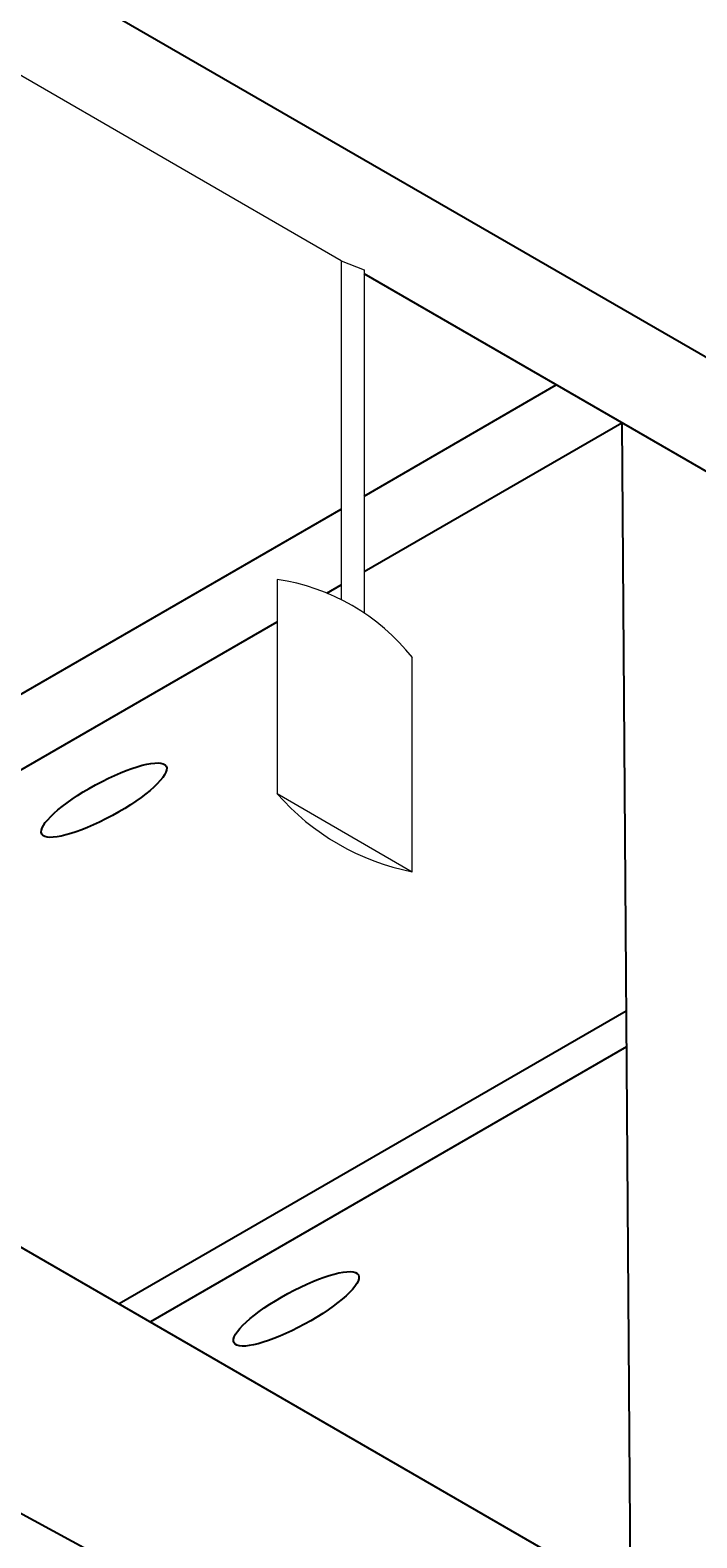
# Model space of a CAD drawing. Units: metres. Extents: x -2391 to 4922, y -635 to 4845.
# Tile 16 of 37: x -1186 to -719, y 1408 to 2464. Entities that reach past the tile are written whole.
import ezdxf

# ---------------------------------------------------------------- set-up
doc = ezdxf.new("R2010")
doc.units = ezdxf.units.M
doc.header["$MEASUREMENT"] = 0
for name, color, linetype, lineweight in [('A-ANNO-DIMS', 2, 'Continuous', 18), ('A-EQPM', 9, 'Continuous', 18), ('A-FLOR-FIXT', 3, 'Continuous', 25)]:
    doc.layers.add(name, color=color, linetype=linetype, lineweight=lineweight)
doc.styles.get("Standard").update_dxf_attribs({"font": 'arial.ttf'})
doc.dimstyles.get("Standard").update_dxf_attribs({"dimtxt": 5, "dimasz": 4, "dimexe": 0.18, "dimexo": 0.0625, "dimgap": 0.09, "dimtad": 0, "dimtih": 1, "dimtoh": 1, "dimdec": 0, "dimzin": 0, "dimdsep": 46, "dimtxsty": 'Standard', "dimcen": 0.09, "dimadec": 0, "dimazin": 0, "dimtfac": 1, "dimtdec": 0, "dimtofl": 0, "dimtmove": 0, "dimatfit": 3, "dimfxl": 1, "dimtolj": 1, "dimtzin": 0, "dimarcsym": 0})

# ---------------------------------------------------------------- blocks, each defined once
blk = doc.blocks.new('UTENSIL-HANGING')
for p, q in [((0, 204.5), (0, 54.7)), ((94.7, 0), (94.7, 149.8)), ((0, 54.7), (94.7, 0))]:
    blk.add_line(p, q)
for centre, radius, start, end in [((-21.4, 58), 148.1, 38.3202, 81.6798), ((126.8, 165), 168.1, 221.0072, 258.9928)]:
    blk.add_arc(centre, radius, start, end)
blk = doc.blocks.new('*D8')
at = {"layer": 'A-ANNO-DIMS', "color": 0, "lineweight": -2, "transparency": 16777216}
for p, q in [((-2047.3, 3005.2), (-2047.3, -631.4)), ((4577.8, 2350.2), (4577.8, -631.4)), ((-2043.3, -631.2), (1257.6, -631.2)), ((4573.8, -631.2), (1272.8, -631.2))]:
    blk.add_line(p, q, dxfattribs=at)
at = {"layer": 'A-ANNO-DIMS', "color": 0, "transparency": 16777216}
for points in [[(-2043.3, -630.6), (-2043.3, -631.9), (-2047.3, -631.2)], [(4573.8, -630.6), (4573.8, -631.9), (4577.8, -631.2)]]:
    blk.add_solid(points, dxfattribs=at)
at = {"layer": 'Defpoints', "color": 0, "transparency": 16777216}
for p in [(-2047.3, 3005.3), (4577.8, 2350.3), (4577.8, -631.2)]:
    blk.add_point(p, dxfattribs=at)
at = {"layer": 'A-ANNO-DIMS', "color": 0, "transparency": 16777216, "insert": (1265.2, -631.2), "char_height": 5, "attachment_point": 5}
blk.add_mtext('\\A1;6625', dxfattribs=at)
blk = doc.blocks.new('*D10')
at = {"layer": 'A-ANNO-DIMS', "color": 0, "lineweight": -2, "transparency": 16777216}
for p, q in [((550.7, 4505.3), (-2384, 4505.3)), ((-2383.8, 4501.3), (-2383.8, 2107.9)), ((-2383.8, -290.7), (-2383.8, 2102.6)), ((-488.6, -294.7), (-2384, -294.7))]:
    blk.add_line(p, q, dxfattribs=at)
at = {"layer": 'A-ANNO-DIMS', "color": 0, "transparency": 16777216}
for points in [[(-2384.5, 4501.3), (-2383.2, 4501.3), (-2383.8, 4505.3)], [(-2384.5, -290.7), (-2383.2, -290.7), (-2383.8, -294.7)]]:
    blk.add_solid(points, dxfattribs=at)
at = {"layer": 'Defpoints', "color": 0, "transparency": 16777216}
for p in [(-2383.8, 4505.3), (550.7, 4505.3), (-488.5, -294.7)]:
    blk.add_point(p, dxfattribs=at)
at = {"layer": 'A-ANNO-DIMS', "color": 0, "transparency": 16777216, "insert": (-2383.8, 2105.3), "char_height": 5, "attachment_point": 5}
blk.add_mtext('\\A1;4800', dxfattribs=at)
blk = doc.blocks.new('*D41')
at = {"layer": 'A-ANNO-DIMS', "color": 0, "lineweight": -2, "transparency": 16777216}
for p, q in [((-2047.3, 3005.3), (-1879, 3296.8)), ((-1875.6, 3294.7), (-1104.2, 2849.3)), ((-323.7, 2398.7), (-1095.1, 2844.1)), ((-488.5, 2105.3), (-320.1, 2396.8))]:
    blk.add_line(p, q, dxfattribs=at)
at = {"layer": 'A-ANNO-DIMS', "color": 0, "transparency": 16777216}
for points in [[(-1875.3, 3295.3), (-1876, 3294.1), (-1879.1, 3296.7)], [(-323.4, 2399.3), (-324, 2398.1), (-320.2, 2396.7)]]:
    blk.add_solid(points, dxfattribs=at)
at = {"layer": 'Defpoints', "color": 0, "transparency": 16777216}
for p in [(-2047.3, 3005.3), (-320.2, 2396.7), (-488.5, 2105.3)]:
    blk.add_point(p, dxfattribs=at)
at = {"layer": 'A-ANNO-DIMS', "color": 0, "transparency": 16777216, "insert": (-1099.7, 2846.7), "char_height": 5, "attachment_point": 5}
blk.add_mtext('\\A1;1800', dxfattribs=at)
blk = doc.blocks.new('*D46')
at = {"layer": 'A-ANNO-DIMS', "color": 0, "lineweight": -2, "transparency": 16777216}
for p, q in [((-2047.3, 1505.3), (-1887.1, 1801.4)), ((-1883.7, 1799.3), (-1087.4, 1368.5)), ((-281.2, 932.4), (-1077.6, 1363.2)), ((-437.8, 634.6), (-277.6, 930.6))]:
    blk.add_line(p, q, dxfattribs=at)
at = {"layer": 'A-ANNO-DIMS', "color": 0, "transparency": 16777216}
for points in [[(-1883.4, 1799.9), (-1884, 1798.7), (-1887.2, 1801.2)], [(-280.9, 933), (-281.6, 931.8), (-277.7, 930.5)]]:
    blk.add_solid(points, dxfattribs=at)
at = {"layer": 'Defpoints', "color": 0, "transparency": 16777216}
for p in [(-2047.3, 1505.3), (-277.7, 930.5), (-437.8, 634.5)]:
    blk.add_point(p, dxfattribs=at)
at = {"layer": 'A-ANNO-DIMS', "color": 0, "transparency": 16777216, "insert": (-1082.5, 1365.9), "char_height": 5, "attachment_point": 5}
blk.add_mtext('\\A1;1830', dxfattribs=at)

msp = doc.modelspace()

# ---------------------------------------------------------------- linework, layer by layer
at = {"layer": 'A-EQPM'}
for p, q in [((-968.1457, 2302.2064), (-1224.8889, 2450.4372)), ((-968.1457, 2302.2064), (-952.2504, 2295.8247)), ((-968.1457, 2302.2064), (-968.1457, 2064.9504)), ((-952.2504, 2295.8247), (-952.2504, 2055.6923))]:
    msp.add_line(p, q, dxfattribs=at)
at = {"layer": 'A-FLOR-FIXT'}
for p, q in [((-2047.3343, 3005.2763), (-488.4886, 2105.2763)), ((-661.9459, 2125.4219), (-952.2504, 2293.0293)), ((-952.2504, 2137.5232), (-817.5782, 2215.2763)), ((-952.2504, 2084.6103), (-771.7543, 2188.8198)), ((-771.7543, 2188.8198), (-765.6167, 1365.2763)), ((-1527.7191, 1805.2763), (-968.1457, 2128.3461)), ((-978.293, 2069.5746), (-968.1457, 2075.4331)), ((-1481.8951, 1778.8198), (-1013.1504, 2049.4496)), ((-1527.7191, 1805.2763), (31.1266, 905.2763)), ((-768.6855, 1777.048), (-1123.7559, 1572.048)), ((-768.4978, 1751.8655), (-1101.8533, 1559.4026))]:
    msp.add_line(p, q, dxfattribs=at)
for centre in [(-1134.366, 1924.6504), (-999.7528, 1568.5473)]:
    msp.add_ellipse(centre, major_axis=(43.5598, 23.7449), ratio=0.246682778, dxfattribs=at)

# ---------------------------------------------------------------- block references
at = {"layer": 'A-EQPM'}
msp.add_blockref('UTENSIL-HANGING', (-1013.1506, 1874.5932), dxfattribs=at)

# ---------------------------------------------------------------- dimensions: what is measured, and where the dimension line sits
at = {"layer": 'A-ANNO-DIMS'}
for base, p1, p2, angle, picture, middle in [((-2383.8343, 4505.2763), (-488.4886, -294.7237), (550.7419, 4505.2763), 90, '*D10', (-2383.8343, 2105.2763)), ((-320.2386, 2396.6938), (-2047.3343, 3005.2763), (-488.4886, 2105.2763), 330, '*D41', (-1099.6615, 2846.6938)), ((-277.7211, 930.4802), (-2047.3343, 1505.2763), (-437.841, 634.5176), 331.5859855, '*D46', (-1082.4677, 1365.8595))]:
    dim = msp.add_linear_dim(base=base, p1=p1, p2=p2, angle=angle, dimstyle='Standard', override={"dimdec": 0, "dimlfac": 1, "dimrnd": 0, "dimzin": 0, "dimdsep": 46, "dimlunit": 2}, dxfattribs=at)
    dim.commit()
    dim.dimension.update_dxf_attribs({"geometry": picture, "text_midpoint": middle})
dim = msp.add_linear_dim(base=(4577.76, -631.2237), p1=(-2047.3343, 3005.2763), p2=(4577.76, 2350.2763), dimstyle='Standard', override={"dimdec": 0, "dimlfac": 1, "dimrnd": 0, "dimzin": 0, "dimdsep": 46, "dimlunit": 2}, dxfattribs=at)
dim.commit()
dim.dimension.update_dxf_attribs({"geometry": '*D8', "text_midpoint": (1265.2128, -631.2237)})

doc.saveas('drawing.dxf')
